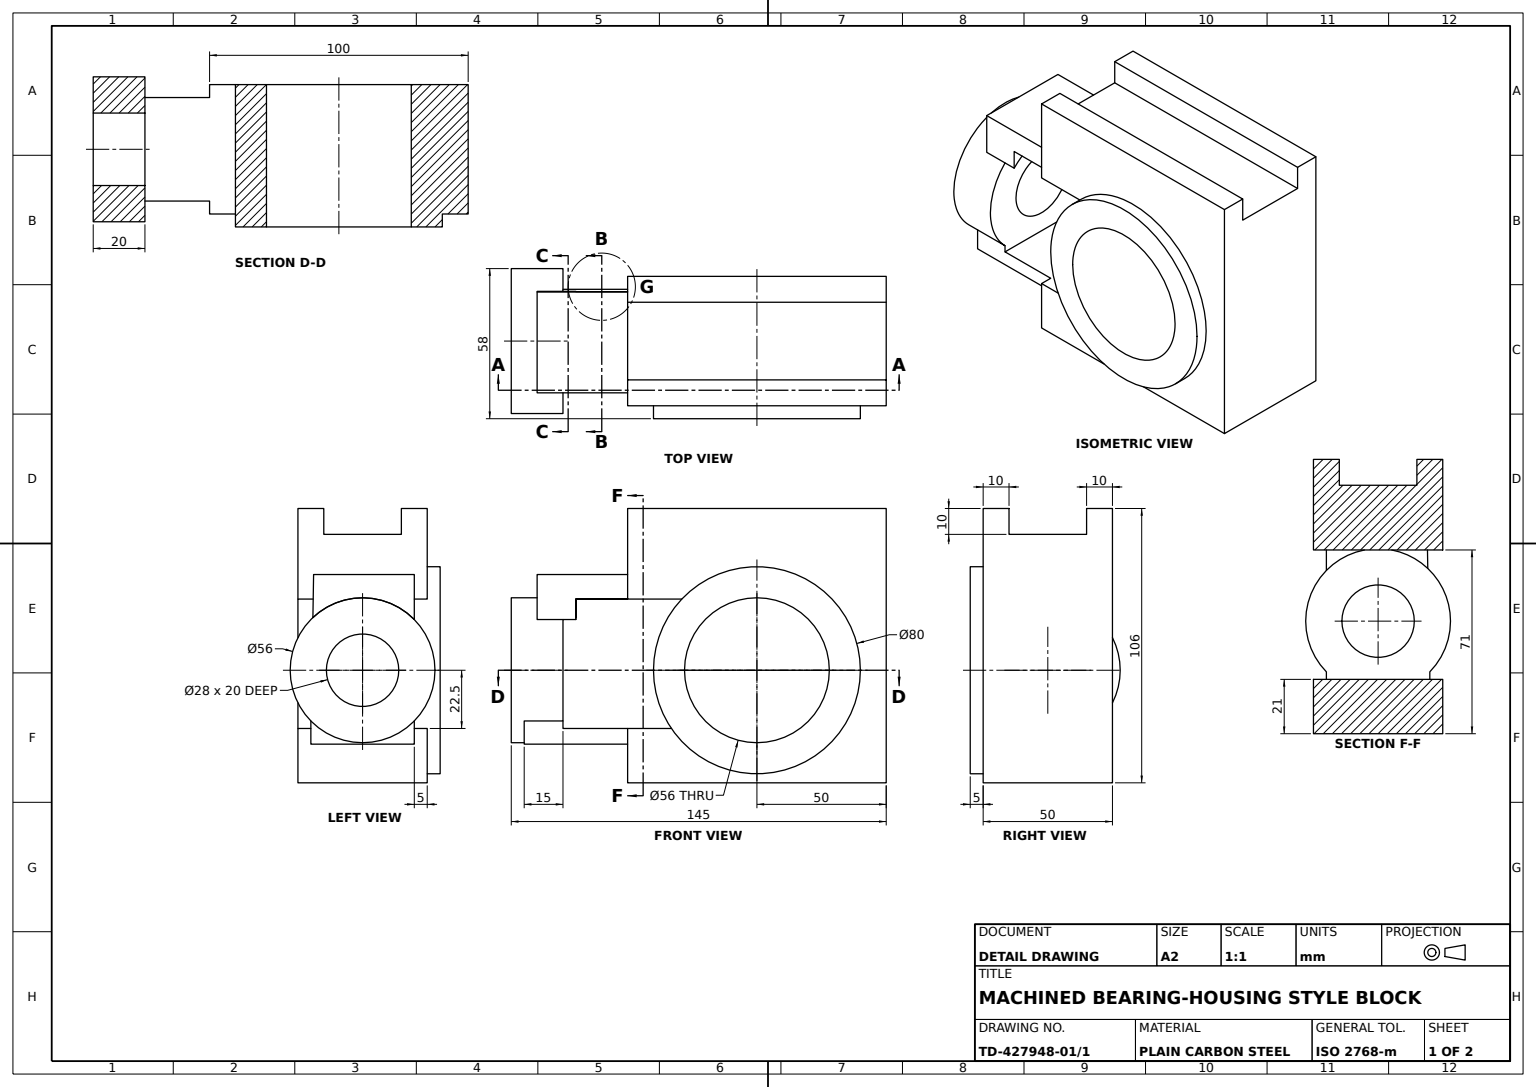
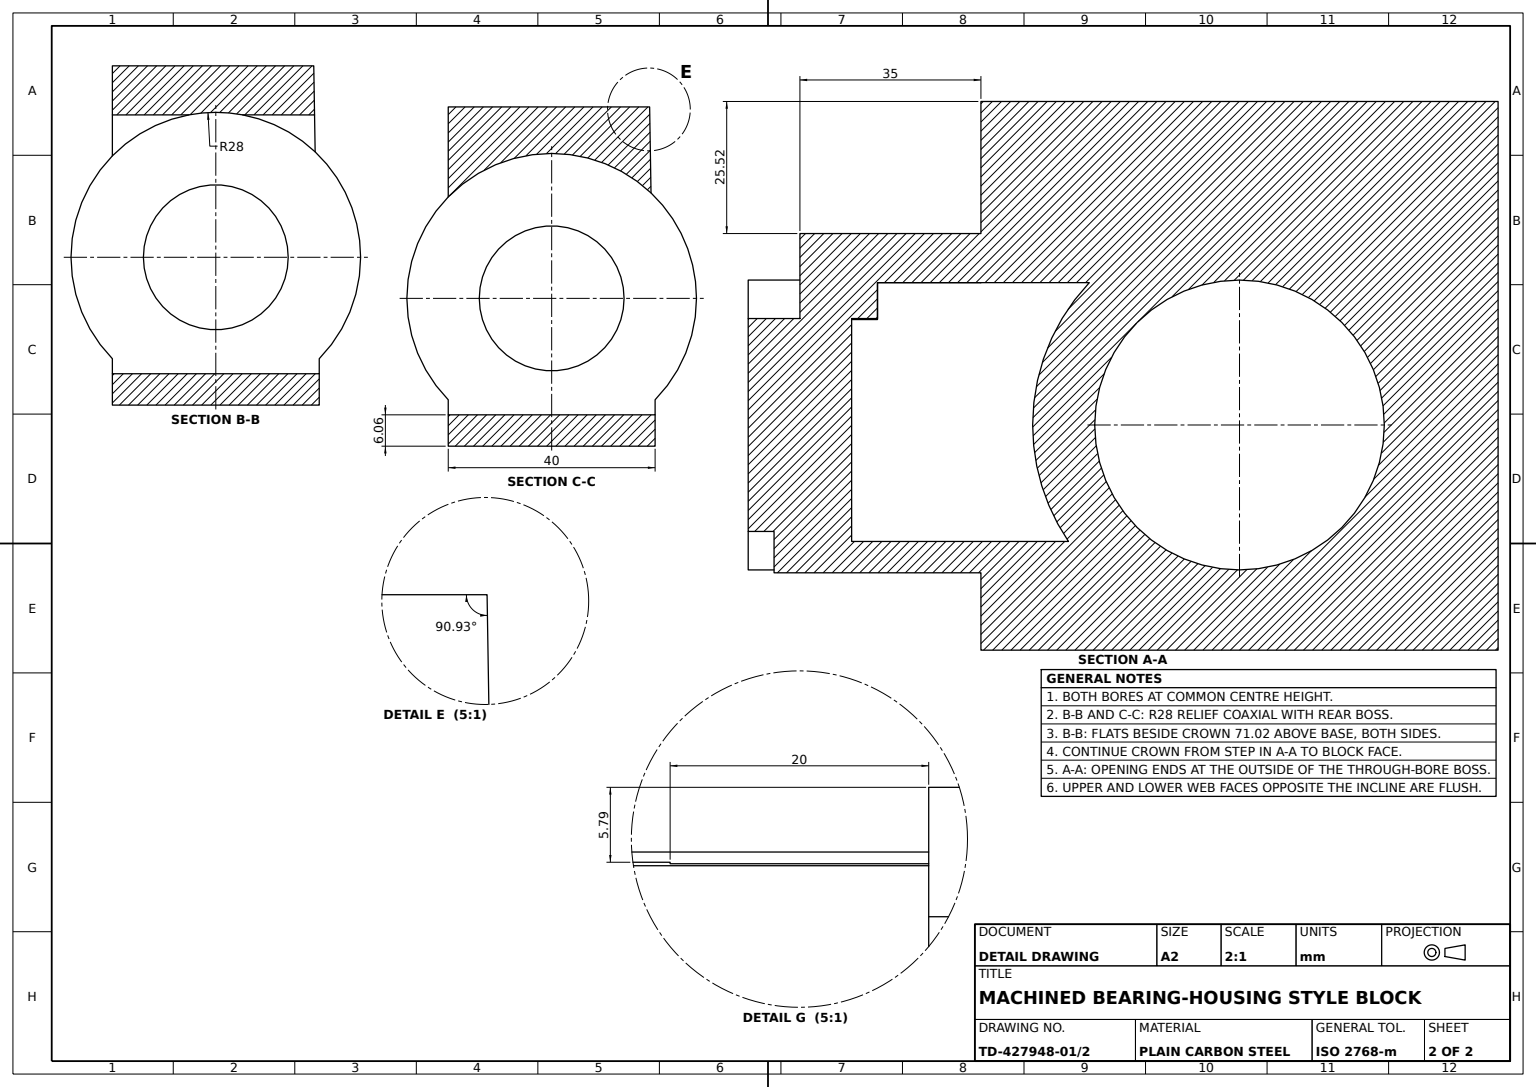
SolidWorks part; units mm, degrees
material "Plain Carbon Steel"
ref_plane "Front Plane" through (0, 0, 0) normal (0, 0, 1) x (1, 0, 0)
ref_plane "Top Plane" through (0, 0, 0) normal (0, 1, 0) x (1, 0, 0)
ref_plane "Right Plane" through (0, 0, 0) normal (1, 0, 0) x (0, 0, -1)
sketch "Base Plate Sketch" plane through (0, 0, 0) normal (0, 1, 0) x (1, 0, 0)
  line L0 (-50, 25) -> (-50, -25)
  line L1 (-50, -25) -> (50, -25)
  line L2 (50, -25) -> (50, 25)
  line L3 (50, 25) -> (-50, 25)
  line L4 (-50, 25) -> (50, -25) construction
  line L5 (-50, -25) -> (50, 25) construction
  point P2 (0, 0)
  dimension "D1" = 100
  dimension "D2" = 50
extrude "Base Plate" add sketch "Base Plate Sketch" along normal blind 21
sketch "Side Web Sketch" plane through (-50, 0, 0) normal (-1, 0, 0) x (0, 0, 1)
  line L0 (-20, 21) -> (-20, 14.9432)
  line L1 (-25, 21) -> (25, 21) construction
  line L2 (-20, 14.9432) -> (20, 14.9432)
  line L3 (20, 14.9432) -> (20, 21)
  line L4 (20, 21) -> (-20, 21)
  line L5 (25, 21) -> (25, 0) construction
  line L6 (-25, 21) -> (-25, 0) construction
  dimension "D1" = 5
  dimension "D2" = 5
  dimension "D3" = 6.0568
extrude "Side Web" add sketch "Side Web Sketch" along normal blind 40
sketch "Rear Bore Boss Sketch" plane through (-90, 0, 0) normal (-1, 0, 0) x (0, 0, 1)
  line L0 (-20, 21) -> (-20, 14.9432) construction
  line L1 (20, 21) -> (-20, 21) construction
  circle A2 centre (0, 43.5) radius 28
  circle A3 centre (0, 43.5) radius 14
  dimension "D1" = 56
  dimension "D3" = 28
  dimension "D2" = 22.5
  dimension "D4" = 20
extrude "Rear Bore Boss" add sketch "Rear Bore Boss Sketch" along normal blind 5 and the other way blind 15
sketch "Front Bore Boss Sketch" plane through (0, 0, 25) normal (0, 0, 1) x (1, 0, 0)
  line L0 (-50, 21) -> (50, 21) construction
  line L1 (50, 21) -> (50, 0) construction
  circle A0 centre (0, 43.5) radius 40
  circle A1 centre (0, 43.5) radius 28
  dimension "D1" = 80
  dimension "D3" = 56
  dimension "D2" = 22.5
  dimension "D4" = 50
extrude "Front Bore Boss" add sketch "Front Bore Boss Sketch" along normal blind 5 and the other way blind 50
sketch "Front Bore Sketch" plane through (0, 0, 30) normal (0, 0, 1) x (1, 0, 0)
  circle A0 centre (0, 43.5) radius 28
  dimension "D1" = 56
extrude "Front Bore" cut sketch "Front Bore Sketch" against normal up to next
sketch "Upright Wall Sketch" plane through (0, 0, 25) normal (0, 0, 1) x (1, 0, 0)
  line L0 (50, 21) -> (50, 106)
  line L1 (50, 106) -> (-50, 106)
  line L2 (-50, 106) -> (-50, 71)
  line L3 (-50, 71) -> (-29.0474, 71)
  line L4 (-50, 0) -> (50, 0) construction
  line L5 (50, 21) -> (33.0719, 21)
  line L6 (33.0719, 21) -> (50, 21) construction
  circle A1 centre (0, 43.5) radius 40 construction
  arc A2 (33.0719, 21) -> (-29.0474, 71) centre (0, 43.5) ccw
  dimension "D1" = 106
  dimension "D2" = 100
  dimension "D3" = 35
extrude "Upright Wall" add sketch "Upright Wall Sketch" against normal blind 50
sketch "Top Slot Sketch" plane through (50, 0, 0) normal (1, 0, 0) x (0, 0, -1)
  line L0 (-15, 106) -> (-15, 96)
  line L1 (25, 106) -> (-25, 106) construction
  line L2 (-15, 96) -> (15, 96)
  line L3 (15, 96) -> (15, 106)
  line L4 (25, 106) -> (25, 0) construction
  line L5 (-25, 106) -> (-25, 0) construction
  dimension "D1" = 10
  dimension "D2" = 10
  dimension "D3" = 10
extrude "Top Slot 10x10" cut sketch "Top Slot Sketch" against normal blind 132 and the other way through all
sketch "Rear Block Sketch" plane through (-50, 0, 0) normal (-1, 0, 0) x (0, 0, 1)
  line L0 (-25, 106) -> (-25, 71) construction
  line L1 (-25, 106) -> (-15, 106) construction
  line L2 (-18.9415, 80.4843) -> (-19.2098, 63.8712)
  line L7 (20, 80.4843) -> (-18.9415, 80.4843)
  line L9 (20, 63.0959) -> (20, 80.4843)
  arc A2 (20, 63.0959) -> (-19.2098, 63.8712) centre (0, 43.5) ccw
  dimension "D1" = 28
  dimension "D2" = 5.7902
  dimension "D3" = 6.0585
  dimension "D4" = 45
  dimension "D5" = 25.5157
extrude "Rear Block" add sketch "Rear Block Sketch" along normal blind 35
sketch "Rear Bore Cut Sketch" plane through (-50, 0, 0) normal (1, 0, 0) x (0, 0, -1)
  line L0 (-20, 71) -> (-20, 63.0959)
  line L2 (19.2098, 63.8712) -> (19.0946, 71)
  line L4 (-20, 71) -> (-5.1929, 71.0142)
  line L5 (19.0946, 71) -> (5.1929, 71.0142)
  arc A0 (19.2098, 63.8712) -> (5.1929, 71.0142) centre (0, 43.5) ccw
  arc A2 (-5.1929, 71.0142) -> (-20, 63.0959) centre (0, 43.5) ccw
  dimension "D1" = 14.0169
extrude "Rear Bore Cut" cut sketch "Rear Bore Cut Sketch" against normal blind 20
sketch "Rear Lug Sketch" plane through (-90, 0, 0) normal (-1, 0, 0) x (0, 0, 1)
  line L0 (-20, 14.9432) -> (-20, 23.9041)
  line L4 (20, 14.9432) -> (20, 23.9041)
  line L5 (-20, 14.9432) -> (20, 14.9432)
  circle A2 centre (0, 43.5) radius 28 construction
  arc A3 (-20, 23.9041) -> (20, 23.9041) centre (0, 43.5) ccw
extrude "Rear Lug" add sketch "Rear Lug Sketch" against normal blind 15
